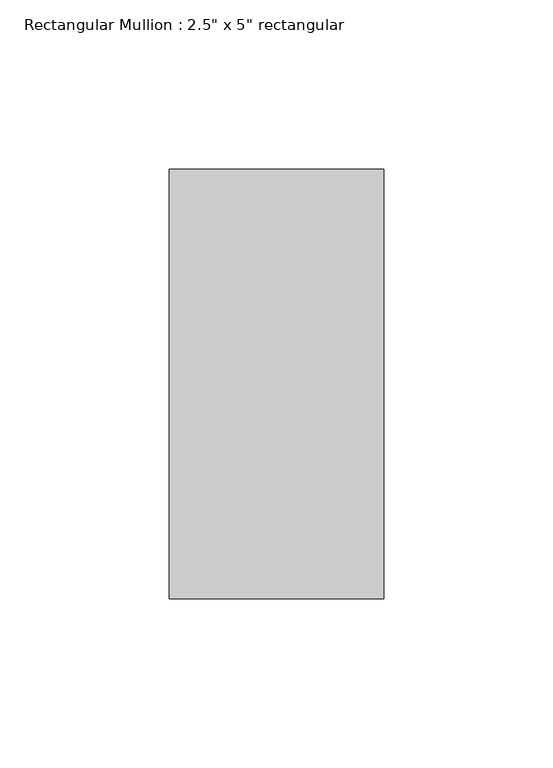
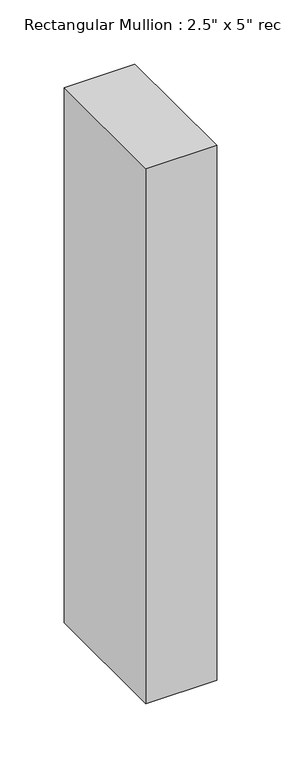
"""IFC4 building model written with IfcOpenShell, lengths in millimetres: member geometry."""

from ifc_helpers import new_model, si_unit, frame, origin, place, context, project, spatial, polyline, outline, extrude, source, transform, mapped, element, save


def member_90750a43(model_context):
    return source(origin(), model_context, "Body", "SweptSolid", [
        extrude(outline(polyline([(31.75, 63.5), (31.75, -63.5), (-31.75, -63.5), (-31.75, 63.5), (31.75, 63.5)])), frame((0.0, 0.0, -508.0), z_axis=(0.0, 0.0, 1.0), x_axis=(1.0, 0.0, 0.0)), (0.0, 0.0, 1.0), 508.0),
    ])


if __name__ == "__main__":
    model = new_model("IFC4")
    model_context = context("Model", 3, world=origin())
    ifc_project = project(units=[si_unit("LENGTHUNIT", "METRE", prefix="MILLI")], contexts=[model_context])
    site = spatial("IfcSite", under=ifc_project)
    building = spatial("IfcBuilding", under=site)
    placement = place(None, origin())
    member_shape = member_90750a43(model_context)
    element("IfcMember", 1, ObjectType="Rectangular Mullion : 2.5\" x 5\" rectangular", at=placement, inside=building, context=model_context, shape_type="MappedRepresentation", body=[
        mapped(member_shape, transform((0.0, 0.0, 0.0), x_axis=(1.0, 0.0, 0.0), y_axis=(0.0, 1.0, 0.0), z_axis=(0.0, 0.0, 1.0))),
    ])
    save(model, "model.ifc")

# Revit data of these elements
# Type "Rectangular Mullion : 2.5\" x 5\" rectangular"
#   built-in parameter 1007304 = 0.416667 (stored number, unit not read)
#   built-in parameter 1007301 = 0.104167 (stored number, unit not read)
#   built-in parameter 1007300 = 0.104167 (stored number, unit not read)
